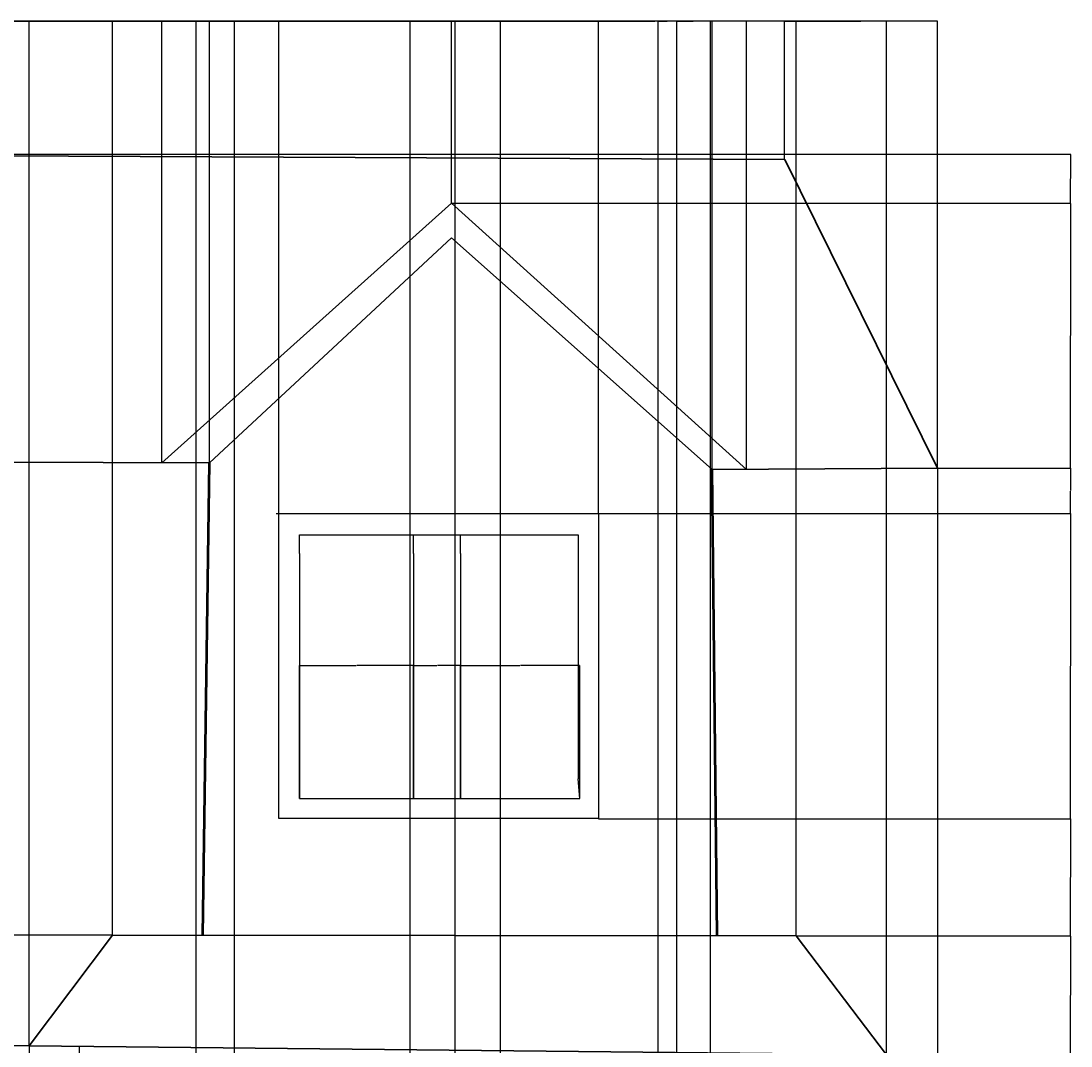
# Model space of a CAD drawing. Units: millimetres. Extents: x 1119 to 4262, y 854 to 2737.
# Tile 5 of 5: x 3118 to 4262, y 1620 to 2737. Entities that reach past the tile are written whole.
import ezdxf

# ---------------------------------------------------------------- set-up
doc = ezdxf.new("R2010")
doc.units = ezdxf.units.MM
for name, color, linetype, lineweight in [('A-ANNO-DIMS', 2, 'Continuous', 18), ('A-GLAZ', 4, 'Continuous', 25), ('A-ROOF', 1, 'Continuous', 35), ('A-WALL', 7, 'Continuous', 50)]:
    doc.layers.add(name, color=color, linetype=linetype, lineweight=lineweight)
doc.styles.get("Standard").update_dxf_attribs({"font": 'arial.ttf'})
doc.dimstyles.get("Standard").update_dxf_attribs({"dimtxt": 0.18, "dimasz": 0.18, "dimexe": 0.18, "dimexo": 0.0625, "dimgap": 0.09, "dimtad": 0, "dimtih": 1, "dimtoh": 1, "dimdec": 4, "dimzin": 0, "dimdsep": 46, "dimtxsty": 'Standard', "dimcen": 0.09, "dimadec": 0, "dimazin": 0, "dimtfac": 1, "dimtdec": 4, "dimtofl": 0, "dimtmove": 0, "dimatfit": 3, "dimfxl": 1, "dimtolj": 1, "dimtzin": 0, "dimarcsym": 0})

# ---------------------------------------------------------------- blocks, each defined once
blk = doc.blocks.new('*D12')
at = {"layer": 'A-ANNO-DIMS', "color": 0, "lineweight": -2, "transparency": 16777216}
for p, q in [((4116.8, 2249.7), (4116.8, 854.2)), ((4000.5, 999.3), (4000.5, 854.2)), ((4000.7, 854.4), (4058.2, 854.4)), ((4116.6, 854.4), (4059.1, 854.4))]:
    blk.add_line(p, q, dxfattribs=at)
at = {"layer": 'A-ANNO-DIMS', "color": 0, "transparency": 16777216}
for points in [[(4000.7, 854.4), (4000.7, 854.3), (4000.5, 854.4)], [(4116.6, 854.4), (4116.6, 854.3), (4116.8, 854.4)]]:
    blk.add_solid(points, dxfattribs=at)
at = {"layer": 'Defpoints', "color": 0, "transparency": 16777216}
for p in [(4116.8, 2249.7), (4000.5, 999.4), (4116.8, 854.4)]:
    blk.add_point(p, dxfattribs=at)
at = {"layer": 'A-ANNO-DIMS', "color": 0, "transparency": 16777216, "insert": (4058.7, 854.4), "char_height": 0.18, "attachment_point": 5}
blk.add_mtext('\\A1;116.25', dxfattribs=at)
blk = doc.blocks.new('*D13')
at = {"layer": 'A-ANNO-DIMS', "color": 0, "lineweight": -2, "transparency": 16777216}
for p, q in [((1264.4, 1028.3), (1264.4, 2737.1)), ((1264.5, 2737), (2690.1, 2737)), ((4116.6, 2737), (2691, 2737)), ((4116.8, 2249.8), (4116.8, 2737.1))]:
    blk.add_line(p, q, dxfattribs=at)
at = {"layer": 'A-ANNO-DIMS', "color": 0, "transparency": 16777216}
for points in [[(1264.5, 2737), (1264.5, 2736.9), (1264.4, 2737)], [(4116.6, 2737), (4116.6, 2736.9), (4116.8, 2737)]]:
    blk.add_solid(points, dxfattribs=at)
at = {"layer": 'Defpoints', "color": 0, "transparency": 16777216}
for p in [(4116.8, 2737), (4116.8, 2249.7), (1264.4, 1028.2)]:
    blk.add_point(p, dxfattribs=at)
at = {"layer": 'A-ANNO-DIMS', "color": 0, "transparency": 16777216, "insert": (2690.6, 2737), "char_height": 0.18, "attachment_point": 5}
blk.add_mtext('\\A1;2852.4', dxfattribs=at)
blk = doc.blocks.new('*D15')
at = {"layer": 'A-ANNO-DIMS', "color": 0, "lineweight": -2, "transparency": 16777216}
for p, q in [((2669.6, 2592), (2669.6, 2737.1)), ((2669.8, 2737), (3309.4, 2737)), ((3949.9, 2737), (3310.3, 2737)), ((3950, 2586.1), (3950, 2737.1))]:
    blk.add_line(p, q, dxfattribs=at)
at = {"layer": 'A-ANNO-DIMS', "color": 0, "transparency": 16777216}
for points in [[(2669.8, 2737), (2669.8, 2736.9), (2669.6, 2737)], [(3949.9, 2737), (3949.9, 2736.9), (3950, 2737)]]:
    blk.add_solid(points, dxfattribs=at)
at = {"layer": 'Defpoints', "color": 0, "transparency": 16777216}
for p in [(3950, 2737), (2669.6, 2592), (3950, 2586)]:
    blk.add_point(p, dxfattribs=at)
at = {"layer": 'A-ANNO-DIMS', "color": 0, "transparency": 16777216, "insert": (3309.8, 2737), "char_height": 0.18, "attachment_point": 5}
blk.add_mtext('\\A1;1280.4', dxfattribs=at)
blk = doc.blocks.new('*D16')
at = {"layer": 'A-ANNO-DIMS', "color": 0, "lineweight": -2, "transparency": 16777216}
for p, q in [((3950, 2586.1), (3950, 2737.1)), ((3950.2, 2737), (4033, 2737)), ((4116.6, 2737), (4033.9, 2737)), ((4116.8, 2249.8), (4116.8, 2737.1))]:
    blk.add_line(p, q, dxfattribs=at)
at = {"layer": 'A-ANNO-DIMS', "color": 0, "transparency": 16777216}
for points in [[(3950.2, 2737), (3950.2, 2736.9), (3950, 2737)], [(4116.6, 2737), (4116.6, 2736.9), (4116.8, 2737)]]:
    blk.add_solid(points, dxfattribs=at)
at = {"layer": 'Defpoints', "color": 0, "transparency": 16777216}
for p in [(4116.8, 2737), (3950, 2586), (4116.8, 2249.7)]:
    blk.add_point(p, dxfattribs=at)
at = {"layer": 'A-ANNO-DIMS', "color": 0, "transparency": 16777216, "insert": (4033.4, 2737), "char_height": 0.18, "attachment_point": 5}
blk.add_mtext('\\A1;166.75', dxfattribs=at)
blk = doc.blocks.new('*D17')
at = {"layer": 'A-ANNO-DIMS', "color": 0, "lineweight": -2, "transparency": 16777216}
for p, q in [((3271.1, 2255.7), (3271.1, 2737.1)), ((3271.3, 2737), (3428.4, 2737)), ((3586.5, 2737), (3429.3, 2737)), ((3586.7, 2538.5), (3586.7, 2737.1))]:
    blk.add_line(p, q, dxfattribs=at)
at = {"layer": 'A-ANNO-DIMS', "color": 0, "transparency": 16777216}
for points in [[(3271.3, 2737), (3271.3, 2736.9), (3271.1, 2737)], [(3586.5, 2737), (3586.5, 2736.9), (3586.7, 2737)]]:
    blk.add_solid(points, dxfattribs=at)
at = {"layer": 'Defpoints', "color": 0, "transparency": 16777216}
for p in [(3586.7, 2737), (3586.7, 2538.4), (3271.1, 2255.7)]:
    blk.add_point(p, dxfattribs=at)
at = {"layer": 'A-ANNO-DIMS', "color": 0, "transparency": 16777216, "insert": (3428.9, 2737), "char_height": 0.18, "attachment_point": 5}
blk.add_mtext('\\A1;315.54', dxfattribs=at)
blk = doc.blocks.new('*D18')
at = {"layer": 'A-ANNO-DIMS', "color": 0, "lineweight": -2, "transparency": 16777216}
for p, q in [((3586.7, 2538.5), (3586.7, 2737.1)), ((3586.8, 2737), (3747.1, 2737)), ((3908.2, 2737), (3748, 2737)), ((3908.4, 2248.4), (3908.4, 2737.1))]:
    blk.add_line(p, q, dxfattribs=at)
at = {"layer": 'A-ANNO-DIMS', "color": 0, "transparency": 16777216}
for points in [[(3586.8, 2737), (3586.8, 2736.9), (3586.7, 2737)], [(3908.2, 2737), (3908.2, 2736.9), (3908.4, 2737)]]:
    blk.add_solid(points, dxfattribs=at)
at = {"layer": 'Defpoints', "color": 0, "transparency": 16777216}
for p in [(3908.4, 2737), (3586.7, 2538.4), (3908.4, 2248.4)]:
    blk.add_point(p, dxfattribs=at)
at = {"layer": 'A-ANNO-DIMS', "color": 0, "transparency": 16777216, "insert": (3747.5, 2737), "char_height": 0.18, "attachment_point": 5}
blk.add_mtext('\\A1;321.74', dxfattribs=at)
blk = doc.blocks.new('*D19')
at = {"layer": 'A-ANNO-DIMS', "color": 0, "lineweight": -2, "transparency": 16777216}
for p, q in [((3323, 2255.6), (3323, 2737.1)), ((3323.2, 2737), (3360.5, 2737)), ((3398.5, 2737), (3361.2, 2737)), ((3398.7, 2200.3), (3398.7, 2737.1))]:
    blk.add_line(p, q, dxfattribs=at)
at = {"layer": 'A-ANNO-DIMS', "color": 0, "transparency": 16777216}
for points in [[(3323.2, 2737), (3323.2, 2736.9), (3323, 2737)], [(3398.5, 2737), (3398.5, 2736.9), (3398.7, 2737)]]:
    blk.add_solid(points, dxfattribs=at)
at = {"layer": 'Defpoints', "color": 0, "transparency": 16777216}
for p in [(3398.7, 2737), (3323, 2255.6), (3398.7, 2200.3)]:
    blk.add_point(p, dxfattribs=at)
at = {"layer": 'A-ANNO-DIMS', "color": 0, "transparency": 16777216, "insert": (3360.9, 2737), "char_height": 0.18, "attachment_point": 5}
blk.add_mtext('\\A1;75.64', dxfattribs=at)
blk = doc.blocks.new('*D20')
at = {"layer": 'A-ANNO-DIMS', "color": 0, "lineweight": -2, "transparency": 16777216}
for p, q in [((3398.7, 2200.3), (3398.7, 2737.1)), ((3398.9, 2737), (3572.5, 2737)), ((3746.9, 2737), (3573.3, 2737)), ((3747.1, 2200.3), (3747.1, 2737.1))]:
    blk.add_line(p, q, dxfattribs=at)
at = {"layer": 'A-ANNO-DIMS', "color": 0, "transparency": 16777216}
for points in [[(3398.9, 2737), (3398.9, 2736.9), (3398.7, 2737)], [(3746.9, 2737), (3746.9, 2736.9), (3747.1, 2737)]]:
    blk.add_solid(points, dxfattribs=at)
at = {"layer": 'Defpoints', "color": 0, "transparency": 16777216}
for p in [(3747.1, 2737), (3398.7, 2200.3), (3747.1, 2200.3)]:
    blk.add_point(p, dxfattribs=at)
at = {"layer": 'A-ANNO-DIMS', "color": 0, "transparency": 16777216, "insert": (3572.9, 2737), "char_height": 0.18, "attachment_point": 5}
blk.add_mtext('\\A1;348.4', dxfattribs=at)
blk = doc.blocks.new('*D21')
at = {"layer": 'A-ANNO-DIMS', "color": 0, "lineweight": -2, "transparency": 16777216}
for p, q in [((3747.1, 2200.3), (3747.1, 2737.1)), ((3747.3, 2737), (3808.6, 2737)), ((3870.8, 2737), (3809.5, 2737)), ((3871, 2248.2), (3871, 2737.1))]:
    blk.add_line(p, q, dxfattribs=at)
at = {"layer": 'A-ANNO-DIMS', "color": 0, "transparency": 16777216}
for points in [[(3747.3, 2737), (3747.3, 2736.9), (3747.1, 2737)], [(3870.8, 2737), (3870.8, 2736.9), (3871, 2737)]]:
    blk.add_solid(points, dxfattribs=at)
at = {"layer": 'Defpoints', "color": 0, "transparency": 16777216}
for p in [(3871, 2737), (3871, 2248.1), (3747.1, 2200.3)]:
    blk.add_point(p, dxfattribs=at)
at = {"layer": 'A-ANNO-DIMS', "color": 0, "transparency": 16777216, "insert": (3809, 2737), "char_height": 0.18, "attachment_point": 5}
blk.add_mtext('\\A1;123.95', dxfattribs=at)
blk = doc.blocks.new('*D22')
at = {"layer": 'A-ANNO-DIMS', "color": 0, "lineweight": -2, "transparency": 16777216}
for p, q in [((3421, 1889.5), (3421, 2034.6)), ((3421.1, 2034.4), (3482.8, 2034.4)), ((3545.3, 2034.4), (3483.6, 2034.4)), ((3545.5, 1889.5), (3545.5, 2034.6))]:
    blk.add_line(p, q, dxfattribs=at)
at = {"layer": 'A-ANNO-DIMS', "color": 0, "transparency": 16777216}
for points in [[(3421.1, 2034.5), (3421.1, 2034.4), (3421, 2034.4)], [(3545.3, 2034.5), (3545.3, 2034.4), (3545.5, 2034.4)]]:
    blk.add_solid(points, dxfattribs=at)
at = {"layer": 'Defpoints', "color": 0, "transparency": 16777216}
for p in [(3545.5, 2034.4), (3421, 1889.4), (3545.5, 1889.4)]:
    blk.add_point(p, dxfattribs=at)
at = {"layer": 'A-ANNO-DIMS', "color": 0, "transparency": 16777216, "insert": (3483.2, 2034.4), "char_height": 0.18, "attachment_point": 5}
blk.add_mtext('\\A1;124.5', dxfattribs=at)
blk = doc.blocks.new('*D23')
at = {"layer": 'A-ANNO-DIMS', "color": 0, "lineweight": -2, "transparency": 16777216}
for p, q in [((3545.5, 1889.5), (3545.5, 2034.6)), ((3545.7, 2034.4), (3570.7, 2034.4)), ((3596.6, 2034.4), (3571.5, 2034.4)), ((3596.7, 1889.5), (3596.7, 2034.6))]:
    blk.add_line(p, q, dxfattribs=at)
at = {"layer": 'A-ANNO-DIMS', "color": 0, "transparency": 16777216}
for points in [[(3545.7, 2034.5), (3545.7, 2034.4), (3545.5, 2034.4)], [(3596.6, 2034.5), (3596.6, 2034.4), (3596.7, 2034.4)]]:
    blk.add_solid(points, dxfattribs=at)
at = {"layer": 'Defpoints', "color": 0, "transparency": 16777216}
for p in [(3596.7, 2034.4), (3545.5, 1889.4), (3596.7, 1889.4)]:
    blk.add_point(p, dxfattribs=at)
at = {"layer": 'A-ANNO-DIMS', "color": 0, "transparency": 16777216, "insert": (3571.1, 2034.4), "char_height": 0.18, "attachment_point": 5}
blk.add_mtext('\\A1;51.27', dxfattribs=at)
blk = doc.blocks.new('*D24')
at = {"layer": 'A-ANNO-DIMS', "color": 0, "lineweight": -2, "transparency": 16777216}
for p, q in [((3596.7, 1889.5), (3596.7, 2034.6)), ((3596.9, 2034.4), (3661.3, 2034.4)), ((3726.5, 2034.4), (3662.2, 2034.4)), ((3726.7, 1889.5), (3726.7, 2034.6))]:
    blk.add_line(p, q, dxfattribs=at)
at = {"layer": 'A-ANNO-DIMS', "color": 0, "transparency": 16777216}
for points in [[(3596.9, 2034.5), (3596.9, 2034.4), (3596.7, 2034.4)], [(3726.5, 2034.5), (3726.5, 2034.4), (3726.7, 2034.4)]]:
    blk.add_solid(points, dxfattribs=at)
at = {"layer": 'Defpoints', "color": 0, "transparency": 16777216}
for p in [(3726.7, 2034.4), (3596.7, 1889.4), (3726.7, 1889.4)]:
    blk.add_point(p, dxfattribs=at)
at = {"layer": 'A-ANNO-DIMS', "color": 0, "transparency": 16777216, "insert": (3661.7, 2034.4), "char_height": 0.18, "attachment_point": 5}
blk.add_mtext('\\A1;129.98', dxfattribs=at)
blk = doc.blocks.new('*D39')
at = {"layer": 'A-ANNO-DIMS', "color": 0, "lineweight": -2, "transparency": 16777216}
for p, q in [((3962.6, 1739.8), (4262, 1739.8)), ((4261.8, 1739.6), (4261.8, 1675.2)), ((4261.8, 1610.4), (4261.8, 1674.8)), ((4061.2, 1610.2), (4262, 1610.2))]:
    blk.add_line(p, q, dxfattribs=at)
at = {"layer": 'A-ANNO-DIMS', "color": 0, "transparency": 16777216}
for points in [[(4261.8, 1739.6), (4261.8, 1739.6), (4261.8, 1739.8)], [(4261.8, 1610.4), (4261.8, 1610.4), (4261.8, 1610.2)]]:
    blk.add_solid(points, dxfattribs=at)
at = {"layer": 'Defpoints', "color": 0, "transparency": 16777216}
for p in [(3962.6, 1739.8), (4261.8, 1739.8), (4061.1, 1610.2)]:
    blk.add_point(p, dxfattribs=at)
at = {"layer": 'A-ANNO-DIMS', "color": 0, "transparency": 16777216, "insert": (4261.8, 1675), "char_height": 0.18, "attachment_point": 5}
blk.add_mtext('\\A1;129.59', dxfattribs=at)
blk = doc.blocks.new('*D40')
at = {"layer": 'A-ANNO-DIMS', "color": 0, "lineweight": -2, "transparency": 16777216}
for p, q in [((3747.1, 1867.6), (4262, 1867.6)), ((4261.8, 1867.5), (4261.8, 1803.9)), ((4261.8, 1740), (4261.8, 1803.5)), ((3962.6, 1739.8), (4262, 1739.8))]:
    blk.add_line(p, q, dxfattribs=at)
at = {"layer": 'A-ANNO-DIMS', "color": 0, "transparency": 16777216}
for points in [[(4261.8, 1867.5), (4261.8, 1867.5), (4261.8, 1867.6)], [(4261.8, 1740), (4261.8, 1740), (4261.8, 1739.8)]]:
    blk.add_solid(points, dxfattribs=at)
at = {"layer": 'Defpoints', "color": 0, "transparency": 16777216}
for p in [(3747.1, 1867.6), (4261.8, 1867.6), (3962.6, 1739.8)]:
    blk.add_point(p, dxfattribs=at)
at = {"layer": 'A-ANNO-DIMS', "color": 0, "transparency": 16777216, "insert": (4261.8, 1803.7), "char_height": 0.18, "attachment_point": 5}
blk.add_mtext('\\A1;127.82', dxfattribs=at)
blk = doc.blocks.new('*D41')
at = {"layer": 'A-ANNO-DIMS', "color": 0, "lineweight": -2, "transparency": 16777216}
for p, q in [((3747.1, 2200.3), (4262, 2200.3)), ((4261.8, 2200.1), (4261.8, 2034.1)), ((4261.8, 1867.8), (4261.8, 2033.8)), ((3747.1, 1867.6), (4262, 1867.6))]:
    blk.add_line(p, q, dxfattribs=at)
at = {"layer": 'A-ANNO-DIMS', "color": 0, "transparency": 16777216}
for points in [[(4261.8, 2200.1), (4261.8, 2200.1), (4261.8, 2200.3)], [(4261.8, 1867.8), (4261.8, 1867.8), (4261.8, 1867.6)]]:
    blk.add_solid(points, dxfattribs=at)
at = {"layer": 'Defpoints', "color": 0, "transparency": 16777216}
for p in [(3747.1, 2200.3), (4261.8, 2200.3), (3747.1, 1867.6)]:
    blk.add_point(p, dxfattribs=at)
at = {"layer": 'A-ANNO-DIMS', "color": 0, "transparency": 16777216, "insert": (4261.8, 2034), "char_height": 0.18, "attachment_point": 5}
blk.add_mtext('\\A1;332.64', dxfattribs=at)
blk = doc.blocks.new('*D42')
at = {"layer": 'A-ANNO-DIMS', "color": 0, "lineweight": -2, "transparency": 16777216}
for p, q in [((4116.9, 2249.7), (4262, 2249.7)), ((4261.8, 2249.6), (4261.8, 2225.2)), ((4261.8, 2200.5), (4261.8, 2224.8)), ((3747.1, 2200.3), (4262, 2200.3))]:
    blk.add_line(p, q, dxfattribs=at)
at = {"layer": 'A-ANNO-DIMS', "color": 0, "transparency": 16777216}
for points in [[(4261.8, 2249.6), (4261.8, 2249.6), (4261.8, 2249.7)], [(4261.8, 2200.5), (4261.8, 2200.5), (4261.8, 2200.3)]]:
    blk.add_solid(points, dxfattribs=at)
at = {"layer": 'Defpoints', "color": 0, "transparency": 16777216}
for p in [(4116.8, 2249.7), (4261.8, 2249.7), (3747.1, 2200.3)]:
    blk.add_point(p, dxfattribs=at)
at = {"layer": 'A-ANNO-DIMS', "color": 0, "transparency": 16777216, "insert": (4261.8, 2225), "char_height": 0.18, "attachment_point": 5}
blk.add_mtext('\\A1;49.46', dxfattribs=at)
blk = doc.blocks.new('*D43')
at = {"layer": 'A-ANNO-DIMS', "color": 0, "lineweight": -2, "transparency": 16777216}
for p, q in [((3586.7, 2538.4), (4262, 2538.4)), ((4261.8, 2538.2), (4261.8, 2394.3)), ((4261.8, 2249.9), (4261.8, 2393.9)), ((4116.9, 2249.7), (4262, 2249.7))]:
    blk.add_line(p, q, dxfattribs=at)
at = {"layer": 'A-ANNO-DIMS', "color": 0, "transparency": 16777216}
for points in [[(4261.8, 2538.2), (4261.8, 2538.2), (4261.8, 2538.4)], [(4261.8, 2249.9), (4261.8, 2249.9), (4261.8, 2249.7)]]:
    blk.add_solid(points, dxfattribs=at)
at = {"layer": 'Defpoints', "color": 0, "transparency": 16777216}
for p in [(3586.7, 2538.4), (4261.8, 2538.4), (4116.8, 2249.7)]:
    blk.add_point(p, dxfattribs=at)
at = {"layer": 'A-ANNO-DIMS', "color": 0, "transparency": 16777216, "insert": (4261.8, 2394.1), "char_height": 0.18, "attachment_point": 5}
blk.add_mtext('\\A1;288.66', dxfattribs=at)
blk = doc.blocks.new('*D44')
at = {"layer": 'A-ANNO-DIMS', "color": 0, "lineweight": -2, "transparency": 16777216}
for p, q in [((2669.7, 2592), (4262, 2592)), ((4261.8, 2591.8), (4261.8, 2565.4)), ((4261.8, 2538.6), (4261.8, 2565)), ((3586.7, 2538.4), (4262, 2538.4))]:
    blk.add_line(p, q, dxfattribs=at)
at = {"layer": 'A-ANNO-DIMS', "color": 0, "transparency": 16777216}
for points in [[(4261.8, 2591.8), (4261.8, 2591.8), (4261.8, 2592)], [(4261.8, 2538.6), (4261.8, 2538.6), (4261.8, 2538.4)]]:
    blk.add_solid(points, dxfattribs=at)
at = {"layer": 'Defpoints', "color": 0, "transparency": 16777216}
for p in [(2669.6, 2592), (4261.8, 2592), (3586.7, 2538.4)]:
    blk.add_point(p, dxfattribs=at)
at = {"layer": 'A-ANNO-DIMS', "color": 0, "transparency": 16777216, "insert": (4261.8, 2565.2), "char_height": 0.18, "attachment_point": 5}
blk.add_mtext('\\A1;53.57', dxfattribs=at)
blk = doc.blocks.new('*D45')
at = {"layer": 'A-ANNO-DIMS', "color": 0, "lineweight": -2, "transparency": 16777216}
for p, q in [((3271.1, 2255.7), (3271.1, 2737.1)), ((3271.3, 2737), (3296.7, 2737)), ((3322.9, 2737), (3297.5, 2737)), ((3323, 2255.6), (3323, 2737.1))]:
    blk.add_line(p, q, dxfattribs=at)
at = {"layer": 'A-ANNO-DIMS', "color": 0, "transparency": 16777216}
for points in [[(3271.3, 2737), (3271.3, 2736.9), (3271.1, 2737)], [(3322.9, 2737), (3322.9, 2736.9), (3323, 2737)]]:
    blk.add_solid(points, dxfattribs=at)
at = {"layer": 'Defpoints', "color": 0, "transparency": 16777216}
for p in [(3323, 2737), (3271.1, 2255.7), (3323, 2255.6)]:
    blk.add_point(p, dxfattribs=at)
at = {"layer": 'A-ANNO-DIMS', "color": 0, "transparency": 16777216, "insert": (3297.1, 2737), "char_height": 0.18, "attachment_point": 5}
blk.add_mtext('\\A1;51.92', dxfattribs=at)
blk = doc.blocks.new('*D62')
at = {"layer": 'A-ANNO-DIMS', "color": 0, "lineweight": -2, "transparency": 16777216}
for p, q in [((3126.3, 1620.1), (3126.3, 2737.1)), ((3126.4, 2737), (3171.4, 2737)), ((3217.1, 2737), (3172.2, 2737)), ((3217.3, 1740.6), (3217.3, 2737.1))]:
    blk.add_line(p, q, dxfattribs=at)
at = {"layer": 'A-ANNO-DIMS', "color": 0, "transparency": 16777216}
for points in [[(3126.4, 2737), (3126.4, 2736.9), (3126.3, 2737)], [(3217.1, 2737), (3217.1, 2736.9), (3217.3, 2737)]]:
    blk.add_solid(points, dxfattribs=at)
at = {"layer": 'Defpoints', "color": 0, "transparency": 16777216}
for p in [(3217.3, 2737), (3217.3, 1740.6), (3126.3, 1620.1)]:
    blk.add_point(p, dxfattribs=at)
at = {"layer": 'A-ANNO-DIMS', "color": 0, "transparency": 16777216, "insert": (3171.8, 2737), "char_height": 0.18, "attachment_point": 5}
blk.add_mtext('\\A1;91.03', dxfattribs=at)
blk = doc.blocks.new('*D63')
at = {"layer": 'A-ANNO-DIMS', "color": 0, "lineweight": -2, "transparency": 16777216}
for p, q in [((3217.3, 1740.6), (3217.3, 2737.1)), ((3217.5, 2737), (3589.5, 2737)), ((3962.4, 2737), (3590.3, 2737)), ((3962.6, 1739.9), (3962.6, 2737.1))]:
    blk.add_line(p, q, dxfattribs=at)
at = {"layer": 'A-ANNO-DIMS', "color": 0, "transparency": 16777216}
for points in [[(3217.5, 2737), (3217.5, 2736.9), (3217.3, 2737)], [(3962.4, 2737), (3962.4, 2736.9), (3962.6, 2737)]]:
    blk.add_solid(points, dxfattribs=at)
at = {"layer": 'Defpoints', "color": 0, "transparency": 16777216}
for p in [(3962.6, 2737), (3217.3, 1740.6), (3962.6, 1739.8)]:
    blk.add_point(p, dxfattribs=at)
at = {"layer": 'A-ANNO-DIMS', "color": 0, "transparency": 16777216, "insert": (3589.9, 2737), "char_height": 0.18, "attachment_point": 5}
blk.add_mtext('\\A1;745.3', dxfattribs=at)
blk = doc.blocks.new('*D64')
at = {"layer": 'A-ANNO-DIMS', "color": 0, "lineweight": -2, "transparency": 16777216}
for p, q in [((3962.6, 1739.9), (3962.6, 2737.1)), ((3962.7, 2737), (4011.4, 2737)), ((4060.9, 2737), (4012.2, 2737)), ((4061.1, 1610.3), (4061.1, 2737.1))]:
    blk.add_line(p, q, dxfattribs=at)
at = {"layer": 'A-ANNO-DIMS', "color": 0, "transparency": 16777216}
for points in [[(3962.7, 2737), (3962.7, 2736.9), (3962.6, 2737)], [(4060.9, 2737), (4060.9, 2736.9), (4061.1, 2737)]]:
    blk.add_solid(points, dxfattribs=at)
at = {"layer": 'Defpoints', "color": 0, "transparency": 16777216}
for p in [(4061.1, 2737), (3962.6, 1739.8), (4061.1, 1610.2)]:
    blk.add_point(p, dxfattribs=at)
at = {"layer": 'A-ANNO-DIMS', "color": 0, "transparency": 16777216, "insert": (4011.8, 2737), "char_height": 0.18, "attachment_point": 5}
blk.add_mtext('\\A1;98.53', dxfattribs=at)
blk = doc.blocks.new('*D65')
at = {"layer": 'A-ANNO-DIMS', "color": 0, "lineweight": -2, "transparency": 16777216}
for p, q in [((3126.3, 1620), (3126.3, 854.2)), ((3181, 1619.4), (3181, 854.2)), ((3126.4, 854.4), (3153.2, 854.4)), ((3180.8, 854.4), (3154, 854.4))]:
    blk.add_line(p, q, dxfattribs=at)
at = {"layer": 'A-ANNO-DIMS', "color": 0, "transparency": 16777216}
for points in [[(3126.4, 854.4), (3126.4, 854.3), (3126.3, 854.4)], [(3180.8, 854.4), (3180.8, 854.3), (3181, 854.4)]]:
    blk.add_solid(points, dxfattribs=at)
at = {"layer": 'Defpoints', "color": 0, "transparency": 16777216}
for p in [(3126.3, 1620.1), (3181, 1619.5), (3181, 854.4)]:
    blk.add_point(p, dxfattribs=at)
at = {"layer": 'A-ANNO-DIMS', "color": 0, "transparency": 16777216, "insert": (3153.6, 854.4), "char_height": 0.18, "attachment_point": 5}
blk.add_mtext('\\A1;54.74', dxfattribs=at)
blk = doc.blocks.new('*D67')
at = {"layer": 'A-ANNO-DIMS', "color": 0, "lineweight": -2, "transparency": 16777216}
for p, q in [((3217.2, 1740.6), (1119.2, 1740.6)), ((1119.4, 1740.4), (1119.4, 1680.5)), ((1119.4, 1620.3), (1119.4, 1680.1)), ((3126.2, 1620.1), (1119.2, 1620.1))]:
    blk.add_line(p, q, dxfattribs=at)
at = {"layer": 'A-ANNO-DIMS', "color": 0, "transparency": 16777216}
for points in [[(1119.3, 1740.4), (1119.4, 1740.4), (1119.4, 1740.6)], [(1119.3, 1620.3), (1119.4, 1620.3), (1119.4, 1620.1)]]:
    blk.add_solid(points, dxfattribs=at)
at = {"layer": 'Defpoints', "color": 0, "transparency": 16777216}
for p in [(1119.4, 1740.6), (3217.3, 1740.6), (3126.3, 1620.1)]:
    blk.add_point(p, dxfattribs=at)
at = {"layer": 'A-ANNO-DIMS', "color": 0, "transparency": 16777216, "insert": (1119.4, 1680.3), "char_height": 0.18, "attachment_point": 5}
blk.add_mtext('\\A1;120.48', dxfattribs=at)
blk = doc.blocks.new('*D81')
at = {"layer": 'A-ANNO-DIMS', "color": 0, "lineweight": -2, "transparency": 16777216}
for p, q in [((3308.6, 1110.8), (3308.6, 2737.1)), ((3308.8, 2737), (3329.2, 2737)), ((3350.3, 2737), (3329.9, 2737)), ((3350.4, 1423.5), (3350.4, 2737.1))]:
    blk.add_line(p, q, dxfattribs=at)
at = {"layer": 'A-ANNO-DIMS', "color": 0, "transparency": 16777216}
for points in [[(3308.8, 2737), (3308.8, 2736.9), (3308.6, 2737)], [(3350.3, 2737), (3350.3, 2736.9), (3350.4, 2737)]]:
    blk.add_solid(points, dxfattribs=at)
at = {"layer": 'Defpoints', "color": 0, "transparency": 16777216}
for p in [(3350.4, 2737), (3350.4, 1423.4), (3308.6, 1110.7)]:
    blk.add_point(p, dxfattribs=at)
at = {"layer": 'A-ANNO-DIMS', "color": 0, "transparency": 16777216, "insert": (3329.5, 2737), "char_height": 0.18, "attachment_point": 5}
blk.add_mtext('\\A1;41.8', dxfattribs=at)
blk = doc.blocks.new('*D82')
at = {"layer": 'A-ANNO-DIMS', "color": 0, "lineweight": -2, "transparency": 16777216}
for p, q in [((3350.4, 1423.5), (3350.4, 2737.1)), ((3350.6, 2737), (3470.2, 2737)), ((3590.6, 2737), (3471, 2737)), ((3590.8, 1396.6), (3590.8, 2737.1))]:
    blk.add_line(p, q, dxfattribs=at)
at = {"layer": 'A-ANNO-DIMS', "color": 0, "transparency": 16777216}
for points in [[(3350.6, 2737), (3350.6, 2736.9), (3350.4, 2737)], [(3590.6, 2737), (3590.6, 2736.9), (3590.8, 2737)]]:
    blk.add_solid(points, dxfattribs=at)
at = {"layer": 'Defpoints', "color": 0, "transparency": 16777216}
for p in [(3590.8, 2737), (3350.4, 1423.4), (3590.8, 1396.6)]:
    blk.add_point(p, dxfattribs=at)
at = {"layer": 'A-ANNO-DIMS', "color": 0, "transparency": 16777216, "insert": (3470.6, 2737), "char_height": 0.18, "attachment_point": 5}
blk.add_mtext('\\A1;240.4', dxfattribs=at)
blk = doc.blocks.new('*D83')
at = {"layer": 'A-ANNO-DIMS', "color": 0, "lineweight": -2, "transparency": 16777216}
for p, q in [((3590.8, 1396.6), (3590.8, 2737.1)), ((3591, 2737), (3701.1, 2737)), ((3812.1, 2737), (3702, 2737)), ((3812.3, 1397.6), (3812.3, 2737.1))]:
    blk.add_line(p, q, dxfattribs=at)
at = {"layer": 'A-ANNO-DIMS', "color": 0, "transparency": 16777216}
for points in [[(3591, 2737), (3591, 2736.9), (3590.8, 2737)], [(3812.1, 2737), (3812.1, 2736.9), (3812.3, 2737)]]:
    blk.add_solid(points, dxfattribs=at)
at = {"layer": 'Defpoints', "color": 0, "transparency": 16777216}
for p in [(3812.3, 2737), (3590.8, 1396.6), (3812.3, 1397.5)]:
    blk.add_point(p, dxfattribs=at)
at = {"layer": 'A-ANNO-DIMS', "color": 0, "transparency": 16777216, "insert": (3701.5, 2737), "char_height": 0.18, "attachment_point": 5}
blk.add_mtext('\\A1;221.45', dxfattribs=at)
blk = doc.blocks.new('*D84')
at = {"layer": 'A-ANNO-DIMS', "color": 0, "lineweight": -2, "transparency": 16777216}
for p, q in [((3812.3, 1397.6), (3812.3, 2737.1)), ((3812.5, 2737), (3822, 2737)), ((3832.4, 2737), (3822.8, 2737)), ((3832.6, 1419.5), (3832.6, 2737.1))]:
    blk.add_line(p, q, dxfattribs=at)
at = {"layer": 'A-ANNO-DIMS', "color": 0, "transparency": 16777216}
for points in [[(3812.5, 2737), (3812.5, 2736.9), (3812.3, 2737)], [(3832.4, 2737), (3832.4, 2736.9), (3832.6, 2737)]]:
    blk.add_solid(points, dxfattribs=at)
at = {"layer": 'Defpoints', "color": 0, "transparency": 16777216}
for p in [(3832.6, 2737), (3832.6, 1419.4), (3812.3, 1397.5)]:
    blk.add_point(p, dxfattribs=at)
at = {"layer": 'A-ANNO-DIMS', "color": 0, "transparency": 16777216, "insert": (3822.4, 2737), "char_height": 0.18, "attachment_point": 5}
blk.add_mtext('\\A1;20.32', dxfattribs=at)
blk = doc.blocks.new('*D85')
at = {"layer": 'A-ANNO-DIMS', "color": 0, "lineweight": -2, "transparency": 16777216}
for p, q in [((3832.6, 1419.5), (3832.6, 2737.1)), ((3832.8, 2737), (3850.4, 2737)), ((3868.9, 2737), (3851.3, 2737)), ((3869.1, 1104.4), (3869.1, 2737.1))]:
    blk.add_line(p, q, dxfattribs=at)
at = {"layer": 'A-ANNO-DIMS', "color": 0, "transparency": 16777216}
for points in [[(3832.8, 2737), (3832.8, 2736.9), (3832.6, 2737)], [(3868.9, 2737), (3868.9, 2736.9), (3869.1, 2737)]]:
    blk.add_solid(points, dxfattribs=at)
at = {"layer": 'Defpoints', "color": 0, "transparency": 16777216}
for p in [(3869.1, 2737), (3832.6, 1419.4), (3869.1, 1104.3)]:
    blk.add_point(p, dxfattribs=at)
at = {"layer": 'A-ANNO-DIMS', "color": 0, "transparency": 16777216, "insert": (3850.9, 2737), "char_height": 0.18, "attachment_point": 5}
blk.add_mtext('\\A1;36.526', dxfattribs=at)
blk = doc.blocks.new('*D86')
at = {"layer": 'A-ANNO-DIMS', "color": 0, "lineweight": -2, "transparency": 16777216}
for p, q in [((3541.7, 1246.4), (3541.7, 2737.1)), ((3541.9, 2737), (3590.6, 2737)), ((3640.1, 2737), (3591.4, 2737)), ((3640.2, 1243), (3640.2, 2737.1))]:
    blk.add_line(p, q, dxfattribs=at)
at = {"layer": 'A-ANNO-DIMS', "color": 0, "transparency": 16777216}
for points in [[(3541.9, 2737), (3541.9, 2736.9), (3541.7, 2737)], [(3640.1, 2737), (3640.1, 2736.9), (3640.2, 2737)]]:
    blk.add_solid(points, dxfattribs=at)
at = {"layer": 'Defpoints', "color": 0, "transparency": 16777216}
for p in [(3640.2, 2737), (3541.7, 1246.4), (3640.2, 1242.9)]:
    blk.add_point(p, dxfattribs=at)
at = {"layer": 'A-ANNO-DIMS', "color": 0, "transparency": 16777216, "insert": (3591, 2737), "char_height": 0.18, "attachment_point": 5}
blk.add_mtext('\\A1;98.55', dxfattribs=at)

msp = doc.modelspace()

# ---------------------------------------------------------------- linework, layer by layer
at = {"layer": 'A-GLAZ'}
for p, q in [((3395.5607, 2200.2798), (3747.0701, 2200.2798)), ((3398.6714, 1867.6403), (3398.6714, 2200.2798)), ((3747.0701, 2200.2798), (3747.0701, 1867.6403)), ((3420.9639, 2156.7569), (3420.9639, 2176.9883)), ((3420.9639, 2176.9883), (3724.7477, 2176.9883)), ((3545.4712, 2156.7569), (3545.4712, 2176.9883)), ((3596.739, 2156.7569), (3596.739, 2176.9883)), ((3724.7477, 2176.9883), (3724.9083, 2156.7569)), ((3420.9639, 2156.7569), (3420.9639, 1911.1632)), ((3545.4712, 2156.7569), (3545.4712, 1911.1632)), ((3596.739, 2156.7569), (3596.739, 1911.1632)), ((3724.9083, 2156.7569), (3724.9083, 1911.1632)), ((3420.9639, 1911.1632), (3420.9639, 1889.4413)), ((3545.4712, 1911.1632), (3545.4712, 1889.4413)), ((3596.739, 1911.1632), (3596.739, 1889.4413)), ((3726.7227, 1889.4413), (3724.9083, 1911.1632)), ((3420.9639, 1889.4413), (3726.7227, 1889.4413)), ((3747.0701, 1867.6403), (3398.6714, 1867.6403))]:
    msp.add_line(p, q, dxfattribs=at)
at = {"layer": 'A-ROOF'}
for p, q in [((2669.6107, 2591.9672), (3950.0418, 2586.0154)), ((4116.7957, 2249.7378), (3950.0418, 2586.0154)), ((3271.1155, 2255.6845), (3586.6565, 2538.4005)), ((3586.6565, 2538.4005), (3908.4009, 2248.3822)), ((3323.0337, 2255.5648), (3586.8111, 2500.6148)), ((3586.8111, 2500.6148), (3871.0219, 2248.139)), ((3323.0337, 2255.5648), (2325.6262, 2257.8652)), ((3871.0219, 2248.139), (4116.7957, 2249.7378)), ((3126.2541, 1620.0857), (3217.2823, 1740.5658)), ((3217.2823, 1740.5658), (3962.5635, 1739.8164)), ((3962.5635, 1739.8164), (4061.0895, 1610.2307)), ((4006.9912, 1610.801), (3126.2541, 1620.0857))]:
    msp.add_line(p, q, dxfattribs=at)
at = {"layer": 'A-WALL'}
for p, q in [((3315.6025, 1740.467), (3323.0337, 2255.5648)), ((3876.5304, 1739.9029), (3871.0219, 2248.139))]:
    msp.add_line(p, q, dxfattribs=at)

# ---------------------------------------------------------------- dimensions: what is measured, and where the dimension line sits
at = {"layer": 'A-ANNO-DIMS'}
for base, p1, p2, override, picture, middle in [((4116.7957, 2736.9672), (1264.3595, 1028.2021), (4116.7957, 2249.7378), {"dimdec": 1, "dimlfac": 1, "dimrnd": 0, "dimzin": 0, "dimdsep": 46, "dimlunit": 2}, '*D13', (2690.5776, 2736.9672)), ((3950.0418, 2736.9672), (2669.6107, 2591.9672), (3950.0418, 2586.0154), {"dimdec": 1, "dimlfac": 1, "dimrnd": 0, "dimzin": 0, "dimdsep": 46, "dimlunit": 2}, '*D15', (3309.8263, 2736.9672)), ((3217.2823, 2736.9672), (3126.2541, 1620.0857), (3217.2823, 1740.5658), {"dimdec": 2, "dimlfac": 1, "dimrnd": 0, "dimzin": 0, "dimdsep": 46, "dimlunit": 2}, '*D62', (3171.7682, 2736.9672)), ((3962.5635, 2736.9672), (3217.2823, 1740.5658), (3962.5635, 1739.8164), {"dimdec": 1, "dimlfac": 1, "dimrnd": 0, "dimzin": 0, "dimdsep": 46, "dimlunit": 2}, '*D63', (3589.9229, 2736.9672)), ((3586.6565, 2736.9672), (3271.1155, 2255.6845), (3586.6565, 2538.4005), {"dimdec": 2, "dimlfac": 1, "dimrnd": 0, "dimzin": 0, "dimdsep": 46, "dimlunit": 2}, '*D17', (3428.886, 2736.9672)), ((3323.0337, 2736.9672), (3271.1155, 2255.6845), (3323.0337, 2255.5648), {"dimdec": 2, "dimlfac": 1, "dimrnd": 0, "dimzin": 0, "dimdsep": 46, "dimlunit": 2}, '*D45', (3297.0746, 2736.9672)), ((3350.4459, 2736.9672), (3308.6482, 1110.6901), (3350.4459, 1423.3892), {"dimdec": 1, "dimlfac": 1, "dimrnd": 0, "dimzin": 0, "dimdsep": 46, "dimlunit": 2}, '*D81', (3329.547, 2736.9672)), ((3398.6714, 2736.9672), (3323.0337, 2255.5648), (3398.6714, 2200.2798), {"dimdec": 2, "dimlfac": 1, "dimrnd": 0, "dimzin": 0, "dimdsep": 46, "dimlunit": 2}, '*D19', (3360.8526, 2736.9672)), ((3590.8232, 2736.9672), (3350.4459, 1423.3892), (3590.8232, 1396.5713), {"dimdec": 1, "dimlfac": 1, "dimrnd": 0, "dimzin": 0, "dimdsep": 46, "dimlunit": 2}, '*D82', (3470.6345, 2736.9672)), ((3747.0701, 2736.9672), (3398.6714, 2200.2798), (3747.0701, 2200.2798), {"dimdec": 1, "dimlfac": 1, "dimrnd": 0, "dimzin": 0, "dimdsep": 46, "dimlunit": 2}, '*D20', (3572.8708, 2736.9672)), ((3640.2453, 2736.9672), (3541.6938, 1246.3571), (3640.2453, 1242.9086), {"dimdec": 2, "dimlfac": 1, "dimrnd": 0, "dimzin": 0, "dimdsep": 46, "dimlunit": 2}, '*D86', (3590.9696, 2736.9672)), ((3908.4009, 2736.9672), (3586.6565, 2538.4005), (3908.4009, 2248.3822), {"dimdec": 2, "dimlfac": 1, "dimrnd": 0, "dimzin": 0, "dimdsep": 46, "dimlunit": 2}, '*D18', (3747.5287, 2736.9672)), ((3812.2711, 2736.9672), (3590.8232, 1396.5713), (3812.2711, 1397.4995), {"dimdec": 2, "dimlfac": 1, "dimrnd": 0, "dimzin": 0, "dimdsep": 46, "dimlunit": 2}, '*D83', (3701.5472, 2736.9672)), ((3871.0219, 2736.9672), (3747.0701, 2200.2798), (3871.0219, 2248.139), {"dimdec": 2, "dimlfac": 1, "dimrnd": 0, "dimzin": 0, "dimdsep": 46, "dimlunit": 2}, '*D21', (3809.046, 2736.9672)), ((3832.5892, 2736.9672), (3812.2711, 1397.4995), (3832.5892, 1419.4082), {"dimdec": 2, "dimlfac": 1, "dimrnd": 0, "dimzin": 0, "dimdsep": 46, "dimlunit": 2}, '*D84', (3822.4302, 2736.9672)), ((3869.1151, 2736.9672), (3832.5892, 1419.4082), (3869.1151, 1104.3083), {"dimdec": 3, "dimlfac": 1, "dimrnd": 0, "dimzin": 0, "dimdsep": 46, "dimlunit": 2}, '*D85', (3850.8521, 2736.9672)), ((4116.7957, 2736.9672), (3950.0418, 2586.0154), (4116.7957, 2249.7378), {"dimdec": 2, "dimlfac": 1, "dimrnd": 0, "dimzin": 0, "dimdsep": 46, "dimlunit": 2}, '*D16', (4033.4187, 2736.9672)), ((4061.0895, 2736.9672), (3962.5635, 1739.8164), (4061.0895, 1610.2307), {"dimdec": 2, "dimlfac": 1, "dimrnd": 0, "dimzin": 0, "dimdsep": 46, "dimlunit": 2}, '*D64', (4011.8265, 2736.9672)), ((4116.7957, 854.3572), (4000.5454, 999.3572), (4116.7957, 2249.7378), {"dimdec": 2, "dimlfac": 1, "dimrnd": 0, "dimzin": 0, "dimdsep": 46, "dimlunit": 2}, '*D12', (4058.6705, 854.3572)), ((3545.4712, 2034.4413), (3420.9639, 1889.4413), (3545.4712, 1889.4413), {"dimdec": 1, "dimlfac": 1, "dimrnd": 0, "dimzin": 0, "dimdsep": 46, "dimlunit": 2}, '*D22', (3483.2175, 2034.4413)), ((3596.739, 2034.4413), (3545.4712, 1889.4413), (3596.739, 1889.4413), {"dimdec": 2, "dimlfac": 1, "dimrnd": 0, "dimzin": 0, "dimdsep": 46, "dimlunit": 2}, '*D23', (3571.1051, 2034.4413)), ((3726.7227, 2034.4413), (3596.739, 1889.4413), (3726.7227, 1889.4413), {"dimdec": 2, "dimlfac": 1, "dimrnd": 0, "dimzin": 0, "dimdsep": 46, "dimlunit": 2}, '*D24', (3661.7308, 2034.4413)), ((3180.996, 854.3572), (3126.2541, 1620.0857), (3180.996, 1619.5086), {"dimdec": 2, "dimlfac": 1, "dimrnd": 0, "dimzin": 0, "dimdsep": 46, "dimlunit": 2}, '*D65', (3153.6251, 854.3572))]:
    dim = msp.add_linear_dim(base=base, p1=p1, p2=p2, dimstyle='Standard', override=override, dxfattribs=at)
    dim.commit()
    dim.dimension.update_dxf_attribs({"geometry": picture, "text_midpoint": middle})
for base, p1, p2, picture, middle in [((4261.7957, 2591.9672), (3586.6565, 2538.4005), (2669.6107, 2591.9672), '*D44', (4261.7957, 2565.1838)), ((4261.7957, 2538.4005), (4116.7957, 2249.7378), (3586.6565, 2538.4005), '*D43', (4261.7957, 2394.0692)), ((4261.7957, 2249.7378), (3747.0701, 2200.2798), (4116.7957, 2249.7378), '*D42', (4261.7957, 2225.0088)), ((4261.7957, 2200.2798), (3747.0701, 1867.6403), (3747.0701, 2200.2798), '*D41', (4261.7957, 2033.96)), ((4261.7957, 1867.6403), (3962.5635, 1739.8164), (3747.0701, 1867.6403), '*D40', (4261.7957, 1803.7283)), ((1119.3595, 1740.5658), (3126.2541, 1620.0857), (3217.2823, 1740.5658), '*D67', (1119.3595, 1680.3258)), ((4261.7957, 1739.8164), (4061.0895, 1610.2307), (3962.5635, 1739.8164), '*D39', (4261.7957, 1675.0236))]:
    dim = msp.add_linear_dim(base=base, p1=p1, p2=p2, angle=90, dimstyle='Standard', override={"dimdec": 2, "dimlfac": 1, "dimrnd": 0, "dimzin": 0, "dimdsep": 46, "dimlunit": 2}, dxfattribs=at)
    dim.commit()
    dim.dimension.update_dxf_attribs({"geometry": picture, "text_midpoint": middle})

doc.saveas('drawing.dxf')
